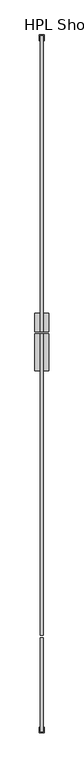
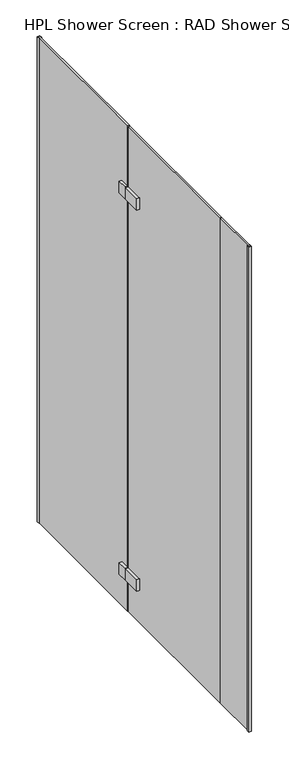
"""IFC4 building model written with IfcOpenShell, lengths in millimetres: flow terminal geometry, HPL Shower Screen : RAD Shower Screen - cut corner."""

from ifc_helpers import new_model, si_unit, frame, origin, origin_with_axes, place, context, project, spatial, polyline, outline, extrude, source, transform, mapped, element, save


def hpl_shower_screen_rad_shower_screen_cut_corner_864de885(model_context):
    return source(origin(), model_context, "Body", "SweptSolid", [
        extrude(outline(polyline([(18.1750129, 0.0), (18.1750129, -650.0), (11.8249871, -650.0), (11.8249871, 0.0), (18.1750129, 0.0)])), origin_with_axes(), (0.0, 0.0, 1.0), 2100.0),
        extrude(outline(polyline([(30.0, 0.0), (30.0, -80.0), (0.0, -80.0), (0.0, 0.0), (30.0, 0.0)])), frame((0.0, 0.0, 140.0), z_axis=(0.0, 0.0, 1.0), x_axis=(1.0, 0.0, 0.0)), (0.0, 0.0, 1.0), 50.0),
        extrude(outline(polyline([(30.0, 0.0), (30.0, -80.0), (0.0, -80.0), (0.0, 0.0), (30.0, 0.0)])), frame((0.0, 0.0, 1790.0), z_axis=(0.0, 0.0, 1.0), x_axis=(1.0, 0.0, 0.0)), (0.0, 0.0, 1.0), 50.0),
        extrude(outline(polyline([(11.8249871, 641.6666667), (18.1750129, 641.6666667), (18.1750129, 4.0), (11.8249871, 4.0), (11.8249871, 641.6666667)])), origin_with_axes(), (0.0, 0.0, 1.0), 2100.0),
        extrude(outline(polyline([(0.0, 44.0), (30.0, 44.0), (30.0, 4.0), (0.0, 4.0), (0.0, 44.0)])), frame((0.0, 0.0, 140.0), z_axis=(0.0, 0.0, 1.0), x_axis=(1.0, 0.0, 0.0)), (0.0, 0.0, 1.0), 50.0),
        extrude(outline(polyline([(0.0, 44.0), (30.0, 44.0), (30.0, 4.0), (0.0, 4.0), (0.0, 44.0)])), frame((0.0, 0.0, 1790.0), z_axis=(0.0, 0.0, 1.0), x_axis=(1.0, 0.0, 0.0)), (0.0, 0.0, 1.0), 50.0),
        extrude(outline(polyline([(11.8249871, -858.3333333), (11.8249871, -655.0), (18.1750129, -655.0), (18.1750129, -858.3333333), (11.8249871, -858.3333333)])), origin_with_axes(), (0.0, 0.0, 1.0), 2100.0),
        extrude(outline(polyline([(11.8249871, 641.6666667), (11.8249871, 631.1666667), (9.8249871, 631.1666667), (9.8249871, 643.6666667), (20.1750129, 643.6666667), (20.1750129, 631.1666667), (18.1750129, 631.1666667), (18.1750129, 641.6666667), (11.8249871, 641.6666667)])), origin_with_axes(), (0.0, 0.0, 1.0), 2100.0),
        extrude(outline(polyline([(11.8249871, -858.3333333), (18.1750129, -858.3333333), (18.1750129, -847.8333333), (20.1750129, -847.8333333), (20.1750129, -860.3333333), (9.8249871, -860.3333333), (9.8249871, -847.8333333), (11.8249871, -847.8333333), (11.8249871, -858.3333333)])), origin_with_axes(), (0.0, 0.0, 1.0), 2100.0),
    ])


if __name__ == "__main__":
    model = new_model("IFC4")
    model_context = context("Model", 3, world=origin())
    ifc_project = project(units=[si_unit("LENGTHUNIT", "METRE", prefix="MILLI")], contexts=[model_context])
    site = spatial("IfcSite", under=ifc_project)
    building = spatial("IfcBuilding", under=site)
    placement = place(None, origin())
    hpl_shower_screen_rad_shower_screen_cut_corner_shape = hpl_shower_screen_rad_shower_screen_cut_corner_864de885(model_context)
    element("IfcFlowTerminal", 1, ObjectType="HPL Shower Screen : RAD Shower Screen - cut corner", at=placement, inside=building, context=model_context, shape_type="MappedRepresentation", body=[
        mapped(hpl_shower_screen_rad_shower_screen_cut_corner_shape, transform((0.0, 0.0, 0.0), x_axis=(1.0, 0.0, 0.0), y_axis=(0.0, 1.0, 0.0), z_axis=(0.0, 0.0, 1.0))),
    ])
    save(model, "model.ifc")

# Revit data of these elements
# Type "HPL Shower Screen : RAD Shower Screen - cut corner"
#   URL = "http://www.matki.co.uk/"
#   Model = "EPW1150 BESPOKE - 'Eauzone Plus' - left hand recess"
#   Manufacturer = "MATKI"
#   Description = "Shower screen - chamfered fixed panel"
#   Fixed panel width [instance default] = 296 mm
#   End Panel Width [instance default] = 100 mm
#   Door Width = 650 mm
#   Offset = 0 mm
#   Height = 2100 mm
#   Door [instance default] = yes
#   Default Elevation = 0
# Element 1 (IfcFlowTerminal, "HPL Shower Screen : RAD Shower Screen - cut corner")
#   Fixed panel width = 637.667 mm
#   End Panel Width = 203.333 mm
#   Materials on its faces: "Metal Joint", "Aluminum 5052", "Glass"
# Materials
#   "Metal Joint": colour RGB 247 247 247, transparency 0
#   "Aluminum 5052": class "Metal", colour RGB 120 120 120, transparency 0, Description = "Aluminum, strain hardened, magnesium alloy, marine", Cost = 0
#   "Glass": class "Glass", colour RGB 0 128 192, transparency 0.9, Description = "Soda Lime Glass", Cost = 0
